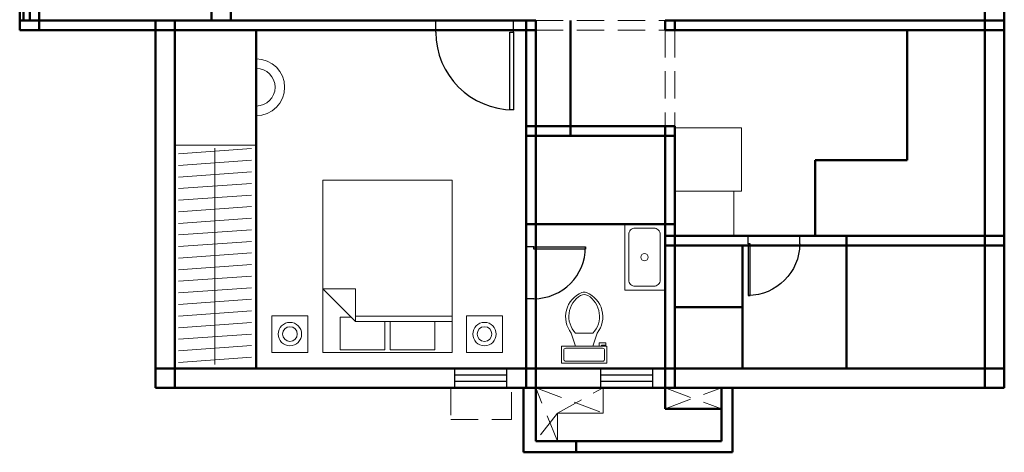
# Model space of a CAD drawing. Units: inches. Extents: x 4795 to 6024, y 2716 to 5025.
# Tile 1 of 19: x 4830 to 5287, y 2716 to 2917. Entities that reach past the tile are written whole.
import ezdxf

# ---------------------------------------------------------------- set-up
doc = ezdxf.new("R2010")
doc.units = ezdxf.units.IN
doc.linetypes.add('DASHED', pattern=[19.05, 12.7, -6.35])
for name, color, linetype, lineweight in [('A-DOOR', 4, 'Continuous', 25), ('A-FLOR-FIXT', 9, 'Continuous', 18), ('A-FURN', 8, 'Continuous', 18), ('A-GLAZ', 4, 'Continuous', 25), ('A-WALL', 7, 'Continuous', 50), ('A-WALL-OVHD', 8, 'DASHED', 18)]:
    doc.layers.add(name, color=color, linetype=linetype, lineweight=lineweight)

# ---------------------------------------------------------------- blocks, each defined once
blk = doc.blocks.new('*U2')
for p, q in [((0, 0), (0, -6)), ((40, 0), (40, -6))]:
    blk.add_line(p, q)
blk.add_lwpolyline([(0, 0), (0, 40), (1.75, 40), (1.75, 0)], close=True)
blk.add_arc((0, 0), 40, 0, 90)
blk = doc.blocks.new('Bed - Queen')
for p, q in [((0, -80.00003), (0, 0)), ((0, 0), (59.99999, 0)), ((59.99999, 0), (59.99999, -80.00003)), ((7.99999, -1.2), (28.79998, -1.2)), ((7.99999, -14.4), (7.99999, -1.2)), ((28.79998, -1.2), (28.79998, -14.4)), ((31.19999, -1.2), (51.99999, -1.2)), ((31.19999, -14.4), (31.19999, -1.2)), ((51.99999, -1.2), (51.99999, -16.4)), ((0, -14.4), (44.8, -14.4)), ((44.8, -16.8), (0, -16.8)), ((59.99999, -29.6), (44.8, -14.4)), ((44.8, -14.4), (44.8, -29.6)), ((51.99999, -16.4), (46.79936, -16.4)), ((44.8, -29.6), (59.99999, -29.6)), ((59.99999, -80.00003), (0, -80.00003))]:
    blk.add_line(p, q)
blk = doc.blocks.new('Toilet - top')
for p, q in [((9.5, -6), (9.5, -2)), ((-10, -8.5), (-8, -8.5)), ((-10, -9.5), (-10, -8.5)), ((-8, -8.5), (-8, -8)), ((-7, -8), (-7, -9.5)), ((-4, -8), (-6, -14)), ((4, -8), (6, -14)), ((-7, -9.5), (-10, -9.5)), ((4, -14), (-4, -14))]:
    blk.add_line(p, q)
blk.add_lwpolyline([(10.5, -8), (10.5, 0), (-10.5, 0), (-10.5, -8)], close=True)
for points in [[(-9.5, -2), (-9.5, -6)], [(8.5, -1), (-8.5, -1)], [(-8.5, -7), (8.5, -7)]]:
    blk.add_lwpolyline(points)
for centre, radius, start, end in [((-8.62, -1.88), 0.884, 81.8699, 188.1301), ((8.62, -1.88), 0.884, 351.8699, 98.1301), ((-8.62, -6.12), 0.884, 171.8699, 278.1301), ((8.62, -6.12), 0.884, 261.8699, 8.1301), ((3.52, -21.58), 12.17, 141.4691, 247.9714), ((4.2, -21.82), 11.33, 136.3677, 238.9468), ((-3.52, -21.58), 12.17, 292.0284, 38.5307), ((-4.2, -21.82), 11.33, 301.053, 43.6321), ((0, -27.88), 4, 245.7318, 294.2682), ((0, -29), 4, 254.8605, 285.1395)]:
    blk.add_arc(centre, radius, start, end)
blk = doc.blocks.new('WIN-24')
for p, q in [((0, 0), (0, 9)), ((0, 9), (24, 9)), ((0, 6), (24, 6)), ((24, 9), (24, 0)), ((24, 3), (0, 3)), ((24, 0), (0, 0))]:
    blk.add_line(p, q)

msp = doc.modelspace()

# ---------------------------------------------------------------- linework, layer by layer
at = {"layer": 'A-FLOR-FIXT'}
msp.add_lwpolyline([(5129.47, 2822.27), (5110.88, 2822.27), (5110.88, 2791.51), (5129.47, 2791.51)], close=True, dxfattribs=at)
msp.add_lwpolyline([(5115.6, 2820.4), (5124.23, 2820.4, -0.414214), (5127.23, 2817.4), (5127.23, 2796.36, -0.414214), (5124.23, 2793.36), (5115.6, 2793.36, -0.414214), (5112.6, 2796.36), (5112.6, 2817.4, -0.414214)], format="xyb", close=True, dxfattribs=at)
msp.add_circle((5119.92, 2806.88), 1.68, dxfattribs=at)
at = {"layer": 'A-FURN'}
for p, q in [((5164.95, 2866.95), (5133.97, 2866.95)), ((5164.95, 2837.52), (5164.95, 2866.95)), ((4901.97, 2858.95), (4939.71, 2858.95)), ((4903.55, 2854.87), (4937.5, 2857.28)), ((4920.52, 2857.46), (4920.52, 2757.03)), ((4903.55, 2849.49), (4937.5, 2851.9)), ((4903.55, 2844.11), (4937.5, 2846.52)), ((4903.55, 2838.73), (4937.5, 2841.14)), ((4903.55, 2833.34), (4937.5, 2835.76)), ((5133.97, 2837.52), (5161.48, 2837.52)), ((5161.48, 2837.52), (5161.48, 2816.74)), ((5161.48, 2837.52), (5164.95, 2837.52)), ((4903.55, 2827.96), (4937.5, 2830.38)), ((4903.55, 2822.58), (4937.5, 2825)), ((4903.55, 2817.2), (4937.5, 2819.62)), ((4903.55, 2811.82), (4937.5, 2814.24)), ((4903.55, 2806.44), (4937.5, 2808.85)), ((4903.55, 2801.06), (4937.5, 2803.47)), ((4903.55, 2795.68), (4937.5, 2798.09)), ((4903.55, 2790.3), (4937.5, 2792.71)), ((4903.55, 2784.92), (4937.5, 2787.33)), ((4903.55, 2779.54), (4937.5, 2781.95)), ((4903.55, 2774.16), (4937.5, 2776.57)), ((4903.55, 2768.77), (4937.5, 2771.19)), ((4903.55, 2763.39), (4937.5, 2765.81)), ((4903.55, 2758.01), (4937.5, 2760.43)), ((5100.74, 2734.49), (5100.74, 2746.24)), ((5079.51, 2721.54), (5079.51, 2734.49)), ((5079.51, 2734.49), (5100.74, 2734.49))]:
    msp.add_line(p, q, dxfattribs=at)
for points in [[(4963.72, 2762.67), (4946.96, 2762.67), (4946.96, 2779.71), (4963.72, 2779.71)], [(5054.04, 2762.68), (5037.28, 2762.68), (5037.28, 2779.72), (5054.04, 2779.72)]]:
    msp.add_lwpolyline(points, close=True, dxfattribs=at)
for centre, radius in [((4955.34, 2771.19), 5.44), ((4955.34, 2771.19), 3.43), ((5045.66, 2771.2), 5.44), ((5045.66, 2771.2), 3.43)]:
    msp.add_circle(centre, radius, dxfattribs=at)
for radius in [13.18, 8.74]:
    msp.add_arc((4939.71, 2885.81), radius, 270, 90, dxfattribs=at)
at = {"layer": 'A-WALL'}
for p, q in [((5277.97, 3359.43), (5277.97, 2746.24)), ((5286.97, 3350.43), (5286.97, 2746.24)), ((4829.88, 3053.24), (4829.88, 2912.24)), ((4831.6, 3052), (4831.6, 2916.74)), ((4834.52, 3050.08), (4834.52, 2916.74)), ((4838.88, 3053.24), (4838.88, 2912.24)), ((4918.88, 3048.74), (4918.88, 2916.74)), ((4927.88, 3048.74), (4927.88, 2916.74)), ((4892.97, 2916.74), (4829.88, 2916.74)), ((4892.97, 2916.74), (4892.97, 2746.24)), ((5069.47, 2916.74), (4892.97, 2916.74)), ((4901.97, 2916.74), (4901.97, 2746.24)), ((5064.97, 2916.74), (5064.97, 2746.24)), ((5069.47, 2916.74), (5069.47, 2746.24)), ((5085.64, 2916.74), (5085.64, 2863.24)), ((5286.97, 2916.74), (5129.47, 2916.74)), ((5129.47, 2916.74), (5129.47, 2912.24)), ((5133.97, 2916.74), (5133.97, 2912.24)), ((4892.97, 2912.24), (4829.88, 2912.24)), ((5069.47, 2912.24), (4892.97, 2912.24)), ((4939.71, 2912.24), (4939.71, 2755.24)), ((5286.97, 2912.24), (5129.47, 2912.24)), ((5241.83, 2852), (5241.83, 2912.24)), ((5133.97, 2867.74), (5064.97, 2867.74)), ((5129.47, 2867.74), (5129.47, 2746.24)), ((5133.97, 2867.74), (5133.97, 2746.24)), ((5133.97, 2863.24), (5064.97, 2863.24)), ((5199.13, 2816.52), (5199.13, 2852)), ((5199.13, 2852), (5241.83, 2852)), ((5064.97, 2822.27), (5133.97, 2822.27)), ((5286.97, 2816.74), (5129.47, 2816.74)), ((5213.7, 2816.74), (5213.7, 2755.24)), ((5286.97, 2812.24), (5129.47, 2812.24)), ((5165.43, 2755.24), (5165.43, 2812.24)), ((5165.43, 2783.74), (5133.97, 2783.74)), ((5286.97, 2755.24), (4892.97, 2755.24)), ((5286.97, 2746.24), (4892.97, 2746.24)), ((5063.73, 2746.24), (5063.73, 2716.3)), ((5069.47, 2746.24), (5069.47, 2721.54)), ((5129.47, 2746.24), (5129.47, 2736.46)), ((5155.61, 2721.54), (5155.61, 2746.24)), ((5160.76, 2716.3), (5160.76, 2746.24)), ((5129.47, 2736.46), (5155.61, 2736.46)), ((5069.47, 2721.54), (5155.61, 2721.54)), ((5088.16, 2721.54), (5088.16, 2716.3)), ((5063.73, 2716.3), (5160.76, 2716.3))]:
    msp.add_line(p, q, dxfattribs=at)
at = {"layer": 'A-WALL-OVHD'}
for p, q in [((5069.47, 2916.74), (5129.47, 2916.74)), ((5069.47, 2912.24), (5129.47, 2912.24)), ((5129.47, 2912.24), (5129.47, 2867.74)), ((5133.97, 2912.24), (5133.97, 2867.74)), ((5030.07, 2746.24), (5030.07, 2731.5)), ((5058.24, 2731.5), (5058.24, 2746.24)), ((5069.47, 2746.24), (5100.74, 2734.49)), ((5079.51, 2721.54), (5069.47, 2746.24)), ((5079.51, 2734.49), (5100.74, 2746.24)), ((5129.47, 2746.24), (5155.61, 2736.46)), ((5129.47, 2736.46), (5155.61, 2746.24)), ((5079.51, 2734.49), (5069.47, 2721.54)), ((5030.07, 2731.5), (5058.24, 2731.5))]:
    msp.add_line(p, q, dxfattribs=at)

# ---------------------------------------------------------------- block references
at = {"layer": 'A-DOOR'}
for p, xscale, yscale, zscale, rotation in [((5059.05, 2911.34), 0.9, 0.9, 0.9, 180), ((5167.99, 2813.14), -0.6, 0.6, 0.6, 180), ((5068.57, 2811.63), 0.6, 0.6, 0.6, 270)]:
    msp.add_blockref('*U2', p, dxfattribs=dict(at, xscale=xscale, yscale=yscale, zscale=zscale, rotation=rotation))
at = {"layer": 'A-FLOR-FIXT', "rotation": 180}
msp.add_blockref('Toilet - top', (5091.94, 2757.61), dxfattribs=at)
at = {"layer": 'A-FURN', "rotation": 180}
msp.add_blockref('Bed - Queen', (5030.64, 2762.67), dxfattribs=at)
at = {"layer": 'A-GLAZ', "rotation": 180}
for p in [(5055.92, 2755.24), (5123.72, 2755.24)]:
    msp.add_blockref('WIN-24', p, dxfattribs=at)

doc.saveas('drawing.dxf')
